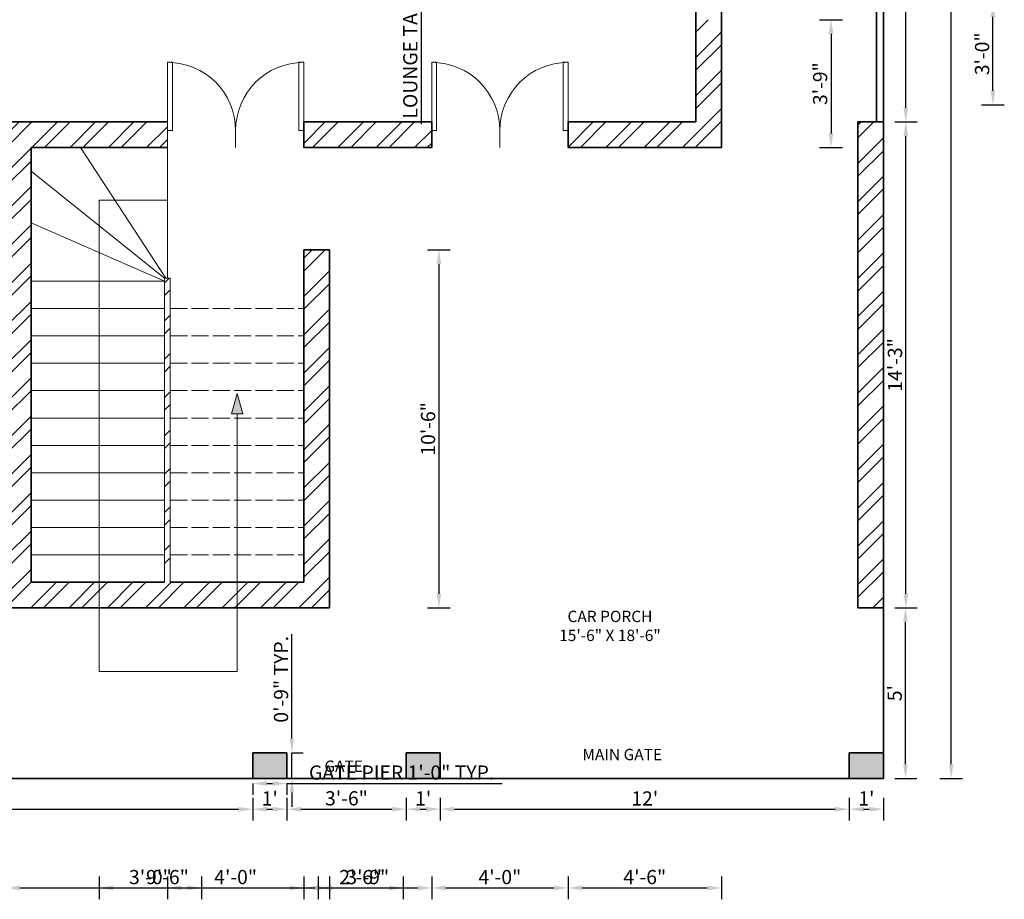
# Model space of a CAD drawing. Units: inches. Extents: x 468 to 1096, y 138 to 946.
# Tile 2 of 6: x 749 to 1096, y 139 to 448. Entities that reach past the tile are written whole.
import ezdxf

# ---------------------------------------------------------------- set-up
doc = ezdxf.new("R2010")
doc.units = ezdxf.units.IN
doc.linetypes.add('ACAD_ISO02W100', pattern=[15, 12, -3])
for name, color, linetype, lineweight in [('A-ANNO-DIMS', 2, 'Continuous', 18), ('A-ANNO-SYMB', 7, 'Continuous', 13), ('A-ANNO-TEXT', 7, 'Continuous', 18), ('A-AREA-IDEN', 7, 'Continuous', 18), ('A-DOOR', 3, 'Continuous', 18), ('A-FLOR-STRS', 7, 'Continuous', 18), ('A-FLOR-STRS-OVHD', 7, 'ACAD_ISO02W100', 18), ('A-SITE-GATE', 7, 'Continuous', 35), ('A-SITE-PATT', 8, 'Continuous', 13), ('A-WALL', 7, 'Continuous', 35), ('A-WALL-PATT', 8, 'Continuous', 13), ('C-PROP', 7, 'Continuous', 35)]:
    doc.layers.add(name, color=color, linetype=linetype, lineweight=lineweight)
doc.styles.get("Standard").update_dxf_attribs({"font": 'arial.ttf'})
doc.dimstyles.new('ISO-25', dxfattribs={"dimtxt": 5, "dimasz": 5, "dimexe": 4, "dimexo": 4, "dimtad": 1, "dimdec": 1, "dimlunit": 3, "dimtxsty": 'Standard', "dimcen": 2.5, "dimadec": 0, "dimazin": 0, "dimtfac": 1, "dimtdec": 1, "dimtmove": 0, "dimatfit": 3, "dimfxl": 4, "dimfxlon": 1, "dimarcsym": 0})

# ---------------------------------------------------------------- blocks, each defined once
blk = doc.blocks.new('*U5')
for p, q in [((-24, 0), (-24, -6)), ((0, 0), (0, -6))]:
    blk.add_line(p, q)
blk.add_lwpolyline([(0, 0), (0, 24), (-1.75, 24), (-1.75, 0)], close=True)
blk.add_arc((0, 0), 24, 90, 180)
blk = doc.blocks.new('*D19')
at = {"layer": 'A-ANNO-DIMS', "color": 0, "lineweight": -2, "transparency": 16777216}
for p, q in [((513.13, 174.32), (513.13, 166.32)), ((831.13, 174.32), (831.13, 166.32)), ((518.13, 170.32), (826.13, 170.32))]:
    blk.add_line(p, q, dxfattribs=at)
at = {"layer": 'A-ANNO-DIMS', "color": 0, "transparency": 16777216}
for points in [[(518.13, 171.15), (518.13, 169.48), (513.13, 170.32)], [(826.13, 171.15), (826.13, 169.48), (831.13, 170.32)]]:
    blk.add_solid(points, dxfattribs=at)
at = {"layer": 'Defpoints', "color": 0, "transparency": 16777216}
for p in [(513.13, 181.16), (831.13, 181.16), (831.13, 170.32)]:
    blk.add_point(p, dxfattribs=at)
at = {"layer": 'A-ANNO-DIMS', "color": 0, "transparency": 16777216, "insert": (672.13, 173.49), "char_height": 5, "attachment_point": 5}
blk.add_mtext('26\'-6"', dxfattribs=at)
blk = doc.blocks.new('*D20')
at = {"layer": 'A-ANNO-DIMS', "color": 0, "lineweight": -2, "transparency": 16777216}
for p, q in [((831.13, 174.32), (831.13, 166.32)), ((843.13, 174.32), (843.13, 166.32)), ((836.13, 170.32), (838.13, 170.32))]:
    blk.add_line(p, q, dxfattribs=at)
at = {"layer": 'A-ANNO-DIMS', "color": 0, "transparency": 16777216}
for points in [[(836.13, 171.15), (836.13, 169.48), (831.13, 170.32)], [(838.13, 171.15), (838.13, 169.48), (843.13, 170.32)]]:
    blk.add_solid(points, dxfattribs=at)
at = {"layer": 'Defpoints', "color": 0, "transparency": 16777216}
for p in [(831.13, 181.16), (843.13, 181.16), (843.13, 170.32)]:
    blk.add_point(p, dxfattribs=at)
at = {"layer": 'A-ANNO-DIMS', "color": 0, "transparency": 16777216, "insert": (837.13, 173.45), "char_height": 5, "attachment_point": 5}
blk.add_mtext("1'", dxfattribs=at)
blk = doc.blocks.new('*D21')
at = {"layer": 'A-ANNO-DIMS', "color": 0, "lineweight": -2, "transparency": 16777216}
for p, q in [((843.13, 174.32), (843.13, 166.32)), ((885.13, 174.32), (885.13, 166.32)), ((848.13, 170.32), (880.13, 170.32))]:
    blk.add_line(p, q, dxfattribs=at)
at = {"layer": 'A-ANNO-DIMS', "color": 0, "transparency": 16777216}
for points in [[(848.13, 171.15), (848.13, 169.48), (843.13, 170.32)], [(880.13, 171.15), (880.13, 169.48), (885.13, 170.32)]]:
    blk.add_solid(points, dxfattribs=at)
at = {"layer": 'Defpoints', "color": 0, "transparency": 16777216}
for p in [(843.13, 181.16), (885.13, 181.16), (885.13, 170.32)]:
    blk.add_point(p, dxfattribs=at)
at = {"layer": 'A-ANNO-DIMS', "color": 0, "transparency": 16777216, "insert": (864.13, 173.5), "char_height": 5, "attachment_point": 5}
blk.add_mtext('3\'-6"', dxfattribs=at)
blk = doc.blocks.new('*D22')
at = {"layer": 'A-ANNO-DIMS', "color": 0, "lineweight": -2, "transparency": 16777216}
for p, q in [((885.13, 174.32), (885.13, 166.32)), ((897.13, 174.32), (897.13, 166.32)), ((890.13, 170.32), (892.13, 170.32))]:
    blk.add_line(p, q, dxfattribs=at)
at = {"layer": 'A-ANNO-DIMS', "color": 0, "transparency": 16777216}
for points in [[(890.13, 171.15), (890.13, 169.48), (885.13, 170.32)], [(892.13, 171.15), (892.13, 169.48), (897.13, 170.32)]]:
    blk.add_solid(points, dxfattribs=at)
at = {"layer": 'Defpoints', "color": 0, "transparency": 16777216}
for p in [(885.13, 181.16), (897.13, 181.16), (897.13, 170.32)]:
    blk.add_point(p, dxfattribs=at)
at = {"layer": 'A-ANNO-DIMS', "color": 0, "transparency": 16777216, "insert": (891.13, 173.45), "char_height": 5, "attachment_point": 5}
blk.add_mtext("1'", dxfattribs=at)
blk = doc.blocks.new('*D23')
at = {"layer": 'A-ANNO-DIMS', "color": 0, "lineweight": -2, "transparency": 16777216}
for p, q in [((897.13, 174.32), (897.13, 166.32)), ((1041.13, 174.32), (1041.13, 166.32)), ((902.13, 170.32), (1036.13, 170.32))]:
    blk.add_line(p, q, dxfattribs=at)
at = {"layer": 'A-ANNO-DIMS', "color": 0, "transparency": 16777216}
for points in [[(902.13, 171.15), (902.13, 169.48), (897.13, 170.32)], [(1036.13, 171.15), (1036.13, 169.48), (1041.13, 170.32)]]:
    blk.add_solid(points, dxfattribs=at)
at = {"layer": 'Defpoints', "color": 0, "transparency": 16777216}
for p in [(897.13, 181.16), (1041.13, 181.16), (1041.13, 170.32)]:
    blk.add_point(p, dxfattribs=at)
at = {"layer": 'A-ANNO-DIMS', "color": 0, "transparency": 16777216, "insert": (969.13, 173.45), "char_height": 5, "attachment_point": 5}
blk.add_mtext("12'", dxfattribs=at)
blk = doc.blocks.new('*D24')
at = {"layer": 'A-ANNO-DIMS', "color": 0, "lineweight": -2, "transparency": 16777216}
for p, q in [((1041.13, 174.32), (1041.13, 166.32)), ((1053.13, 174.32), (1053.13, 166.32)), ((1046.13, 170.32), (1048.13, 170.32))]:
    blk.add_line(p, q, dxfattribs=at)
at = {"layer": 'A-ANNO-DIMS', "color": 0, "transparency": 16777216}
for points in [[(1046.13, 171.15), (1046.13, 169.48), (1041.13, 170.32)], [(1048.13, 171.15), (1048.13, 169.48), (1053.13, 170.32)]]:
    blk.add_solid(points, dxfattribs=at)
at = {"layer": 'Defpoints', "color": 0, "transparency": 16777216}
for p in [(1041.13, 181.16), (1053.13, 181.16), (1053.13, 170.32)]:
    blk.add_point(p, dxfattribs=at)
at = {"layer": 'A-ANNO-DIMS', "color": 0, "transparency": 16777216, "insert": (1047.13, 173.45), "char_height": 5, "attachment_point": 5}
blk.add_mtext("1'", dxfattribs=at)
blk = doc.blocks.new('*D25')
at = {"layer": 'A-ANNO-DIMS', "color": 0, "lineweight": -2, "transparency": 16777216}
for p, q in [((1057.13, 241.16), (1064.91, 241.16)), ((1060.91, 186.16), (1060.91, 236.16)), ((1057.13, 181.16), (1064.91, 181.16))]:
    blk.add_line(p, q, dxfattribs=at)
at = {"layer": 'A-ANNO-DIMS', "color": 0, "transparency": 16777216}
for points in [[(1060.07, 236.16), (1061.74, 236.16), (1060.91, 241.16)], [(1060.07, 186.16), (1061.74, 186.16), (1060.91, 181.16)]]:
    blk.add_solid(points, dxfattribs=at)
at = {"layer": 'Defpoints', "color": 0, "transparency": 16777216}
for p in [(1053.13, 241.16), (1060.91, 241.16), (1053.13, 181.16)]:
    blk.add_point(p, dxfattribs=at)
at = {"layer": 'A-ANNO-DIMS', "color": 0, "transparency": 16777216, "insert": (1057.74, 211.16), "char_height": 5, "attachment_point": 5, "rotation": 90}
blk.add_mtext("5'", dxfattribs=at)
blk = doc.blocks.new('*D26')
at = {"layer": 'A-ANNO-DIMS', "color": 0, "lineweight": -2, "transparency": 16777216}
for p, q in [((1073, 901.16), (1081, 901.16)), ((1077, 186.16), (1077, 896.16)), ((1073, 181.16), (1081, 181.16))]:
    blk.add_line(p, q, dxfattribs=at)
at = {"layer": 'A-ANNO-DIMS', "color": 0, "transparency": 16777216}
for points in [[(1076.17, 896.16), (1077.83, 896.16), (1077, 901.16)], [(1076.17, 186.16), (1077.83, 186.16), (1077, 181.16)]]:
    blk.add_solid(points, dxfattribs=at)
at = {"layer": 'Defpoints', "color": 0, "transparency": 16777216}
for p in [(1053.13, 901.16), (1077, 901.16), (1053.13, 181.16)]:
    blk.add_point(p, dxfattribs=at)
at = {"layer": 'A-ANNO-DIMS', "color": 0, "transparency": 16777216, "insert": (1073.82, 541.16), "char_height": 5, "attachment_point": 5, "rotation": 90}
blk.add_mtext("60'", dxfattribs=at)
blk = doc.blocks.new('*D27')
at = {"layer": 'A-ANNO-DIMS', "color": 0, "lineweight": -2, "transparency": 16777216}
for p, q in [((1057.13, 412.16), (1065.02, 412.16)), ((1061.02, 246.16), (1061.02, 407.16)), ((1057.13, 241.16), (1065.02, 241.16))]:
    blk.add_line(p, q, dxfattribs=at)
at = {"layer": 'A-ANNO-DIMS', "color": 0, "transparency": 16777216}
for points in [[(1060.18, 407.16), (1061.85, 407.16), (1061.02, 412.16)], [(1060.18, 246.16), (1061.85, 246.16), (1061.02, 241.16)]]:
    blk.add_solid(points, dxfattribs=at)
at = {"layer": 'Defpoints', "color": 0, "transparency": 16777216}
for p in [(1053.13, 412.16), (1061.02, 412.16), (1053.13, 241.16)]:
    blk.add_point(p, dxfattribs=at)
at = {"layer": 'A-ANNO-DIMS', "color": 0, "transparency": 16777216, "insert": (1057.84, 326.66), "char_height": 5, "attachment_point": 5, "rotation": 90}
blk.add_mtext('14\'-3"', dxfattribs=at)
blk = doc.blocks.new('*D28')
at = {"layer": 'A-ANNO-DIMS', "color": 0, "lineweight": -2, "transparency": 16777216}
for p, q in [((1057.13, 853.16), (1065.02, 853.16)), ((1061.02, 417.16), (1061.02, 848.16)), ((1057.13, 412.16), (1065.02, 412.16))]:
    blk.add_line(p, q, dxfattribs=at)
at = {"layer": 'A-ANNO-DIMS', "color": 0, "transparency": 16777216}
for points in [[(1060.18, 848.16), (1061.85, 848.16), (1061.02, 853.16)], [(1060.18, 417.16), (1061.85, 417.16), (1061.02, 412.16)]]:
    blk.add_solid(points, dxfattribs=at)
at = {"layer": 'Defpoints', "color": 0, "transparency": 16777216}
for p in [(1053.13, 853.16), (1061.02, 853.16), (1053.13, 412.16)]:
    blk.add_point(p, dxfattribs=at)
at = {"layer": 'A-ANNO-DIMS', "color": 0, "transparency": 16777216, "insert": (1057.84, 632.66), "char_height": 5, "attachment_point": 5, "rotation": 90}
blk.add_mtext('36\'-9"', dxfattribs=at)
blk = doc.blocks.new('GATE-PIER-12X9')
for p, q in [((0, 0), (0, 9)), ((0, 9), (12, 9)), ((12, 9), (12, 0))]:
    blk.add_line(p, q)
blk = doc.blocks.new('*D45')
at = {"layer": 'A-ANNO-DIMS', "color": 0, "lineweight": -2, "transparency": 16777216}
for p, q in [((831.13, 179.36), (831.13, 175.36)), ((836.13, 179.36), (838.13, 179.36)), ((843.13, 179.36), (843.13, 175.36)), ((843.13, 179.36), (918.98, 179.36))]:
    blk.add_line(p, q, dxfattribs=at)
at = {"layer": 'A-ANNO-DIMS', "color": 0, "transparency": 16777216}
for points in [[(836.13, 180.19), (836.13, 178.53), (831.13, 179.36)], [(838.13, 180.19), (838.13, 178.53), (843.13, 179.36)]]:
    blk.add_solid(points, dxfattribs=at)
at = {"layer": 'Defpoints', "color": 0, "transparency": 16777216}
for p in [(831.13, 181.16), (843.13, 181.16), (843.13, 179.36)]:
    blk.add_point(p, dxfattribs=at)
at = {"layer": 'A-ANNO-DIMS', "color": 0, "transparency": 16777216, "insert": (883.55, 182.57), "char_height": 5, "attachment_point": 5}
blk.add_mtext('GATE PIER 1\'-0" TYP.', dxfattribs=at)
blk = doc.blocks.new('*D46')
at = {"layer": 'A-ANNO-DIMS', "color": 0, "lineweight": -2, "transparency": 16777216}
for p, q in [((844.93, 195.16), (844.93, 231.89)), ((844.93, 190.16), (848.93, 190.16)), ((844.93, 181.16), (844.93, 190.16)), ((844.93, 181.16), (848.93, 181.16)), ((844.93, 176.16), (844.93, 171.16))]:
    blk.add_line(p, q, dxfattribs=at)
at = {"layer": 'A-ANNO-DIMS', "color": 0, "transparency": 16777216}
for points in [[(844.1, 195.16), (845.76, 195.16), (844.93, 190.16)], [(844.1, 176.16), (845.76, 176.16), (844.93, 181.16)]]:
    blk.add_solid(points, dxfattribs=at)
at = {"layer": 'Defpoints', "color": 0, "transparency": 16777216}
for p in [(843.13, 190.16), (844.93, 190.16), (843.13, 181.16)]:
    blk.add_point(p, dxfattribs=at)
at = {"layer": 'A-ANNO-DIMS', "color": 0, "transparency": 16777216, "insert": (841.75, 216.03), "char_height": 5, "attachment_point": 5, "rotation": 90}
blk.add_mtext('0\'-9" TYP.', dxfattribs=at)
blk = doc.blocks.new('*D51')
at = {"layer": 'A-ANNO-DIMS', "color": 0, "lineweight": -2, "transparency": 16777216}
for p, q in [((894.45, 546.23), (886.45, 546.23)), ((890.45, 541.23), (890.45, 491.23)), ((894.45, 486.23), (886.45, 486.23)), ((890.45, 486.23), (890.45, 411.4))]:
    blk.add_line(p, q, dxfattribs=at)
at = {"layer": 'A-ANNO-DIMS', "color": 0, "transparency": 16777216}
for points in [[(889.62, 541.23), (891.28, 541.23), (890.45, 546.23)], [(889.62, 491.23), (891.28, 491.23), (890.45, 486.23)]]:
    blk.add_solid(points, dxfattribs=at)
at = {"layer": 'Defpoints', "color": 0, "transparency": 16777216}
for p in [(899.45, 546.23), (890.45, 486.23), (899.45, 486.23)]:
    blk.add_point(p, dxfattribs=at)
at = {"layer": 'A-ANNO-DIMS', "color": 0, "transparency": 16777216, "insert": (887.24, 446.31), "char_height": 5, "attachment_point": 5, "rotation": 90}
blk.add_mtext('LOUNGE TABLE 5\'-0"', dxfattribs=at)
blk = doc.blocks.new('*D55')
at = {"layer": 'A-ANNO-DIMS', "color": 0, "lineweight": -2, "transparency": 16777216}
for p, q in [((744.13, 146.61), (744.13, 138.61)), ((858.13, 146.61), (858.13, 138.61)), ((749.13, 142.61), (853.13, 142.61))]:
    blk.add_line(p, q, dxfattribs=at)
at = {"layer": 'A-ANNO-DIMS', "color": 0, "transparency": 16777216}
for points in [[(749.13, 143.44), (749.13, 141.78), (744.13, 142.61)], [(853.13, 143.44), (853.13, 141.78), (858.13, 142.61)]]:
    blk.add_solid(points, dxfattribs=at)
at = {"layer": 'Defpoints', "color": 0, "transparency": 16777216}
for p in [(744.13, 241.16), (858.13, 241.16), (858.13, 142.61)]:
    blk.add_point(p, dxfattribs=at)
at = {"layer": 'A-ANNO-DIMS', "color": 0, "transparency": 16777216, "insert": (801.13, 145.79), "char_height": 5, "attachment_point": 5}
blk.add_mtext('9\'-6"', dxfattribs=at)
blk = doc.blocks.new('*D56')
at = {"layer": 'A-ANNO-DIMS', "color": 0, "lineweight": -2, "transparency": 16777216}
for p, q in [((892.68, 367.16), (900.68, 367.16)), ((896.68, 362.16), (896.68, 246.16)), ((892.68, 241.16), (900.68, 241.16))]:
    blk.add_line(p, q, dxfattribs=at)
at = {"layer": 'A-ANNO-DIMS', "color": 0, "transparency": 16777216}
for points in [[(895.85, 362.16), (897.51, 362.16), (896.68, 367.16)], [(895.85, 246.16), (897.51, 246.16), (896.68, 241.16)]]:
    blk.add_solid(points, dxfattribs=at)
at = {"layer": 'Defpoints', "color": 0, "transparency": 16777216}
for p in [(858.13, 367.16), (858.13, 241.16), (896.68, 241.16)]:
    blk.add_point(p, dxfattribs=at)
at = {"layer": 'A-ANNO-DIMS', "color": 0, "transparency": 16777216, "insert": (893.5, 304.16), "char_height": 5, "attachment_point": 5, "rotation": 90}
blk.add_mtext('10\'-6"', dxfattribs=at)
blk = doc.blocks.new('*D57')
at = {"layer": 'A-ANNO-DIMS', "color": 0, "lineweight": -2, "transparency": 16777216}
for p, q in [((801.13, 146.61), (801.13, 138.61)), ((849.13, 146.61), (849.13, 138.61)), ((806.13, 142.61), (844.13, 142.61))]:
    blk.add_line(p, q, dxfattribs=at)
at = {"layer": 'A-ANNO-DIMS', "color": 0, "transparency": 16777216}
for points in [[(806.13, 143.44), (806.13, 141.78), (801.13, 142.61)], [(844.13, 143.44), (844.13, 141.78), (849.13, 142.61)]]:
    blk.add_solid(points, dxfattribs=at)
at = {"layer": 'Defpoints', "color": 0, "transparency": 16777216}
for p in [(801.13, 403.16), (849.13, 403.16), (849.13, 142.61)]:
    blk.add_point(p, dxfattribs=at)
at = {"layer": 'A-ANNO-DIMS', "color": 0, "transparency": 16777216, "insert": (825.13, 145.79), "char_height": 5, "attachment_point": 5}
blk.add_mtext('4\'-0"', dxfattribs=at)
blk = doc.blocks.new('*D58')
at = {"layer": 'A-ANNO-DIMS', "color": 0, "lineweight": -2, "transparency": 16777216}
for p, q in [((849.13, 146.61), (849.13, 138.61)), ((894.13, 146.61), (894.13, 138.61)), ((854.13, 142.61), (889.13, 142.61))]:
    blk.add_line(p, q, dxfattribs=at)
at = {"layer": 'A-ANNO-DIMS', "color": 0, "transparency": 16777216}
for points in [[(854.13, 143.44), (854.13, 141.78), (849.13, 142.61)], [(889.13, 143.44), (889.13, 141.78), (894.13, 142.61)]]:
    blk.add_solid(points, dxfattribs=at)
at = {"layer": 'Defpoints', "color": 0, "transparency": 16777216}
for p in [(849.13, 403.16), (894.13, 403.16), (894.13, 142.61)]:
    blk.add_point(p, dxfattribs=at)
at = {"layer": 'A-ANNO-DIMS', "color": 0, "transparency": 16777216, "insert": (871.63, 145.79), "char_height": 5, "attachment_point": 5}
blk.add_mtext('3\'-9"', dxfattribs=at)
blk = doc.blocks.new('*D59')
at = {"layer": 'A-ANNO-DIMS', "color": 0, "lineweight": -2, "transparency": 16777216}
for p, q in [((894.13, 146.61), (894.13, 138.61)), ((942.13, 146.61), (942.13, 138.61)), ((899.13, 142.61), (937.13, 142.61))]:
    blk.add_line(p, q, dxfattribs=at)
at = {"layer": 'A-ANNO-DIMS', "color": 0, "transparency": 16777216}
for points in [[(899.13, 143.44), (899.13, 141.78), (894.13, 142.61)], [(937.13, 143.44), (937.13, 141.78), (942.13, 142.61)]]:
    blk.add_solid(points, dxfattribs=at)
at = {"layer": 'Defpoints', "color": 0, "transparency": 16777216}
for p in [(894.13, 403.16), (942.13, 403.16), (942.13, 142.61)]:
    blk.add_point(p, dxfattribs=at)
at = {"layer": 'A-ANNO-DIMS', "color": 0, "transparency": 16777216, "insert": (918.13, 145.79), "char_height": 5, "attachment_point": 5}
blk.add_mtext('4\'-0"', dxfattribs=at)
blk = doc.blocks.new('*D60')
at = {"layer": 'A-ANNO-DIMS', "color": 0, "lineweight": -2, "transparency": 16777216}
for p, q in [((942.13, 146.61), (942.13, 138.61)), ((996.13, 146.61), (996.13, 138.61)), ((947.13, 142.61), (991.13, 142.61))]:
    blk.add_line(p, q, dxfattribs=at)
at = {"layer": 'A-ANNO-DIMS', "color": 0, "transparency": 16777216}
for points in [[(947.13, 143.44), (947.13, 141.78), (942.13, 142.61)], [(991.13, 143.44), (991.13, 141.78), (996.13, 142.61)]]:
    blk.add_solid(points, dxfattribs=at)
at = {"layer": 'Defpoints', "color": 0, "transparency": 16777216}
for p in [(942.13, 403.16), (996.13, 403.16), (996.13, 142.61)]:
    blk.add_point(p, dxfattribs=at)
at = {"layer": 'A-ANNO-DIMS', "color": 0, "transparency": 16777216, "insert": (969.13, 145.79), "char_height": 5, "attachment_point": 5}
blk.add_mtext('4\'-6"', dxfattribs=at)
blk = doc.blocks.new('*D63')
at = {"layer": 'A-ANNO-DIMS', "color": 0, "lineweight": -2, "transparency": 16777216}
for p, q in [((777.13, 146.61), (777.13, 138.61)), ((813.13, 146.61), (813.13, 138.61)), ((782.13, 142.61), (808.13, 142.61))]:
    blk.add_line(p, q, dxfattribs=at)
at = {"layer": 'A-ANNO-DIMS', "color": 0, "transparency": 16777216}
for points in [[(782.13, 143.44), (782.13, 141.78), (777.13, 142.61)], [(808.13, 143.44), (808.13, 141.78), (813.13, 142.61)]]:
    blk.add_solid(points, dxfattribs=at)
at = {"layer": 'Defpoints', "color": 0, "transparency": 16777216}
for p in [(777.13, 682.16), (813.13, 682.16), (813.13, 142.61)]:
    blk.add_point(p, dxfattribs=at)
at = {"layer": 'A-ANNO-DIMS', "color": 0, "transparency": 16777216, "insert": (795.13, 145.79), "char_height": 5, "attachment_point": 5}
blk.add_mtext('3\'-0"', dxfattribs=at)
blk = doc.blocks.new('*D64')
at = {"layer": 'A-ANNO-DIMS', "color": 0, "lineweight": -2, "transparency": 16777216}
for p, q in [((854.13, 146.61), (854.13, 138.61)), ((884.13, 146.61), (884.13, 138.61)), ((859.13, 142.61), (879.13, 142.61))]:
    blk.add_line(p, q, dxfattribs=at)
at = {"layer": 'A-ANNO-DIMS', "color": 0, "transparency": 16777216}
for points in [[(859.13, 143.44), (859.13, 141.78), (854.13, 142.61)], [(879.13, 143.44), (879.13, 141.78), (884.13, 142.61)]]:
    blk.add_solid(points, dxfattribs=at)
at = {"layer": 'Defpoints', "color": 0, "transparency": 16777216}
for p in [(854.13, 766.16), (884.13, 766.16), (884.13, 142.61)]:
    blk.add_point(p, dxfattribs=at)
at = {"layer": 'A-ANNO-DIMS', "color": 0, "transparency": 16777216, "insert": (869.13, 145.79), "char_height": 5, "attachment_point": 5}
blk.add_mtext('2\'-6"', dxfattribs=at)
blk = doc.blocks.new('*D70')
at = {"layer": 'A-ANNO-DIMS', "color": 0, "lineweight": -2, "transparency": 16777216}
for p, q in [((1030.68, 448.16), (1038.68, 448.16)), ((1034.68, 443.16), (1034.68, 408.16)), ((1030.68, 403.16), (1038.68, 403.16))]:
    blk.add_line(p, q, dxfattribs=at)
at = {"layer": 'A-ANNO-DIMS', "color": 0, "transparency": 16777216}
for points in [[(1033.85, 443.16), (1035.51, 443.16), (1034.68, 448.16)], [(1033.85, 408.16), (1035.51, 408.16), (1034.68, 403.16)]]:
    blk.add_solid(points, dxfattribs=at)
at = {"layer": 'Defpoints', "color": 0, "transparency": 16777216}
for p in [(996.13, 448.16), (996.13, 403.16), (1034.68, 403.16)]:
    blk.add_point(p, dxfattribs=at)
at = {"layer": 'A-ANNO-DIMS', "color": 0, "transparency": 16777216, "insert": (1031.5, 425.66), "char_height": 5, "attachment_point": 5, "rotation": 90}
blk.add_mtext('3\'-9"', dxfattribs=at)
blk = doc.blocks.new('*D76')
at = {"layer": 'A-ANNO-DIMS', "color": 0, "lineweight": -2, "transparency": 16777216}
for p, q in [((1087.68, 454.16), (1095.68, 454.16)), ((1091.68, 423.16), (1091.68, 449.16)), ((1087.68, 418.16), (1095.68, 418.16))]:
    blk.add_line(p, q, dxfattribs=at)
at = {"layer": 'A-ANNO-DIMS', "color": 0, "transparency": 16777216}
for points in [[(1090.85, 449.16), (1092.51, 449.16), (1091.68, 454.16)], [(1090.85, 423.16), (1092.51, 423.16), (1091.68, 418.16)]]:
    blk.add_solid(points, dxfattribs=at)
at = {"layer": 'Defpoints', "color": 0, "transparency": 16777216}
for p in [(687.13, 454.16), (1091.68, 454.16), (687.13, 418.16)]:
    blk.add_point(p, dxfattribs=at)
at = {"layer": 'A-ANNO-DIMS', "color": 0, "transparency": 16777216, "insert": (1088.5, 436.16), "char_height": 5, "attachment_point": 5, "rotation": 90}
blk.add_mtext('3\'-0"', dxfattribs=at)

msp = doc.modelspace()

# ---------------------------------------------------------------- hatches: boundary and pattern name
at = {"layer": 'A-ANNO-SYMB'}
h = msp.add_hatch(color=256, dxfattribs=at)
h.dxf.hatch_style = 1
h.paths.add_polyline_path([(825.63, 316.65), (823.63, 309.43), (825.63, 309.43), (827.63, 309.43)])
at = {"layer": 'A-SITE-PATT'}
h = msp.add_hatch(color=256, dxfattribs=at)
h.dxf.hatch_style = 1
h.paths.add_polyline_path([(731.29, 185.66), (719.29, 185.66), (719.29, 181.16), (731.29, 181.16)])
h.paths.add_polyline_path([(843.13, 190.16), (831.13, 190.16), (831.13, 181.16), (843.13, 181.16)])
h.paths.add_polyline_path([(897.13, 190.16), (885.13, 190.16), (885.13, 181.16), (897.13, 181.16)])
h.paths.add_polyline_path([(1053.13, 190.16), (1041.13, 190.16), (1041.13, 181.16), (1053.13, 181.16)])
at = {"layer": 'A-WALL-PATT'}
h = msp.add_hatch(dxfattribs=at)
h.set_pattern_fill('ANSI32', color=256)
h.paths.add_polyline_path([(1053.13, 412.16), (1044.13, 412.16), (1044.13, 241.16), (1053.13, 241.16)])
h.paths.add_polyline_path([(996.13, 448.16), (987.13, 448.16), (987.13, 412.16), (942.13, 412.16), (942.13, 403.16), (996.13, 403.16)])
h.paths.add_polyline_path([(996.13, 532.16), (987.13, 532.16), (987.13, 496.16), (996.13, 496.16)])
h.paths.add_polyline_path([(996.13, 646.16), (987.13, 646.16), (987.13, 607.16), (813.13, 607.16), (813.13, 598.16), (822.13, 598.16), (987.13, 598.16), (987.13, 592.16), (996.13, 592.16), (996.13, 598.16), (996.13, 607.16)])
h.paths.add_polyline_path([(894.13, 412.16), (849.13, 412.16), (849.13, 403.16), (894.13, 403.16)])
h.paths.add_polyline_path([(801.13, 412.16), (744.13, 412.16), (744.13, 250.16), (744.13, 241.16), (777.13, 241.16), (777.13, 250.16), (753.13, 250.16), (753.13, 403.16), (801.13, 403.16)])
h.paths.add_polyline_path([(744.13, 412.16), (736.13, 412.16), (736.13, 403.16), (744.13, 403.16)])
h = msp.add_hatch(dxfattribs=at)
h.set_pattern_fill('ANSI32', color=256)
h.paths.add_polyline_path([(858.13, 367.16), (849.13, 367.16), (849.13, 250.16), (825.63, 250.16), (825.63, 241.16), (840.13, 241.16), (849.13, 241.16), (858.13, 241.16)])
h.paths.add_polyline_path([(825.63, 250.16), (802.13, 250.16), (802.13, 357.16), (800.13, 357.16), (800.13, 250.16), (777.13, 250.16), (777.13, 241.16), (825.63, 241.16)])

# ---------------------------------------------------------------- linework, layer by layer
at = {"layer": 'A-ANNO-SYMB'}
for p, q in [((801.13, 384.66), (777.13, 384.66)), ((777.13, 384.66), (777.13, 218.74)), ((823.63, 309.43), (825.63, 316.65)), ((827.63, 309.43), (825.63, 316.65)), ((825.63, 309.43), (823.63, 309.43)), ((825.63, 218.74), (825.63, 309.43)), ((825.63, 309.43), (827.63, 309.43)), ((777.13, 218.74), (825.63, 218.74))]:
    msp.add_line(p, q, dxfattribs=at)
at = {"layer": 'A-FLOR-STRS'}
for p, q in [((801.13, 357.16), (801.13, 412.16)), ((800.61, 357.16), (770.53, 403.16)), ((800.13, 357.16), (753.13, 394.88)), ((800.13, 356.16), (753.13, 376.68)), ((800.13, 357.16), (800.13, 250.16)), ((802.13, 357.16), (800.13, 357.16)), ((802.13, 357.16), (802.13, 250.16)), ((800.13, 356.16), (753.13, 356.16)), ((800.13, 346.53), (753.13, 346.53)), ((800.13, 336.89), (753.13, 336.89)), ((800.13, 327.26), (753.13, 327.26)), ((800.13, 317.62), (753.13, 317.62)), ((800.13, 307.98), (753.13, 307.98)), ((800.13, 298.35), (753.13, 298.35)), ((800.13, 288.71), (753.13, 288.71)), ((800.13, 279.08), (753.13, 279.08)), ((800.13, 269.44), (753.13, 269.44)), ((800.13, 259.81), (753.13, 259.81))]:
    msp.add_line(p, q, dxfattribs=at)
at = {"layer": 'A-FLOR-STRS-OVHD', "ltscale": 0.5}
for p, q in [((802.13, 346.53), (849.13, 346.53)), ((802.13, 336.89), (849.13, 336.89)), ((802.13, 327.26), (849.13, 327.26)), ((802.13, 317.62), (849.13, 317.62)), ((802.13, 307.98), (849.13, 307.98)), ((802.13, 298.35), (849.13, 298.35)), ((802.13, 288.71), (849.13, 288.71)), ((802.13, 279.08), (849.13, 279.08)), ((802.13, 269.44), (849.13, 269.44)), ((802.13, 259.81), (849.13, 259.81))]:
    msp.add_line(p, q, dxfattribs=at)
at = {"layer": 'A-SITE-GATE'}
for p, q in [((1041.13, 181.16), (1041.13, 190.16)), ((1041.13, 190.16), (1053.13, 190.16))]:
    msp.add_line(p, q, dxfattribs=at)
at = {"layer": 'A-WALL'}
for p, q in [((987.13, 412.16), (987.13, 598.16)), ((996.13, 403.16), (996.13, 598.16)), ((744.13, 412.16), (801.13, 412.16)), ((849.13, 412.16), (894.13, 412.16)), ((849.13, 403.16), (849.13, 412.16)), ((894.13, 403.16), (894.13, 412.16)), ((942.13, 403.16), (942.13, 412.16)), ((942.13, 412.16), (987.13, 412.16)), ((753.13, 403.16), (753.13, 250.16)), ((753.13, 403.16), (801.13, 403.16)), ((849.13, 403.16), (894.13, 403.16)), ((942.13, 403.16), (996.13, 403.16)), ((849.13, 250.16), (849.13, 367.16)), ((849.13, 367.16), (858.13, 367.16)), ((858.13, 241.16), (858.13, 367.16)), ((753.13, 250.16), (800.13, 250.16)), ((802.13, 250.16), (849.13, 250.16)), ((744.13, 241.16), (840.13, 241.16)), ((840.13, 241.16), (849.13, 241.16)), ((849.13, 241.16), (858.13, 241.16))]:
    msp.add_line(p, q, dxfattribs=at)
at = {"layer": 'C-PROP'}
for p, q in [((1053.13, 181.16), (1053.13, 901.16)), ((1050.72, 412.16), (1050.72, 892.16)), ((1044.13, 241.16), (1044.13, 412.16)), ((1044.13, 412.16), (1053.13, 412.16)), ((1044.13, 241.16), (1053.13, 241.16)), ((513.13, 181.16), (1053.13, 181.16))]:
    msp.add_line(p, q, dxfattribs=at)

# ---------------------------------------------------------------- block references
at = {"layer": 'A-DOOR', "xscale": -1}
for p in [(801.13, 409.16), (894.13, 409.16)]:
    msp.add_blockref('*U5', p, dxfattribs=at)
at = {"layer": 'A-DOOR'}
for p in [(849.13, 409.16), (942.13, 409.16)]:
    msp.add_blockref('*U5', p, dxfattribs=at)
at = {"layer": 'A-SITE-GATE'}
for p in [(831.13, 181.16), (885.13, 181.16)]:
    msp.add_blockref('GATE-PIER-12X9', p, dxfattribs=at)

# ---------------------------------------------------------------- texts
at = {"layer": 'A-ANNO-TEXT', "char_height": 4, "attachment_point": 1}
for s, insert in [('\\pxqc;MAIN GATE', (943.07, 191.56)), ('\\pxqc;GATE', (845.02, 187.44))]:
    msp.add_mtext_dynamic_manual_height_columns(s, width=36.2598, gutter_width=12.5, heights=[0], dxfattribs=dict(at, insert=insert))
at = {"layer": 'A-AREA-IDEN', "insert": (938.75, 240.16), "char_height": 4, "attachment_point": 1}
msp.add_mtext_dynamic_manual_height_columns('\\pxqc;CAR PORCH\\P15\'-6" X 18\'-6"', width=36.2598, gutter_width=12.5, heights=[0], dxfattribs=at)

# ---------------------------------------------------------------- dimensions: what is measured, and where the dimension line sits
at = {"layer": 'A-ANNO-DIMS'}
for base, p1, p2, angle, override, picture, middle in [((1077, 901.16), (1053.13, 181.16), (1053.13, 901.16), 90, {"dimclrd": 0, "dimclre": 0, "dimclrt": 0}, '*D26', (1073.82, 541.16)), ((1061.02, 853.16), (1053.13, 412.16), (1053.13, 853.16), 90, {"dimclrd": 0, "dimclre": 0, "dimclrt": 0}, '*D28', (1057.84, 632.66)), ((1091.68, 454.16), (687.13, 418.16), (687.13, 454.16), 90, {"dimdec": 1, "dimlfac": 1, "dimrnd": 0, "dimzin": 1, "dimdsep": 46, "dimlunit": 4, "dimfrac": 2}, '*D76', (1088.5, 436.16)), ((1034.68, 403.16), (996.13, 448.16), (996.13, 403.16), 270, {"dimdec": 1, "dimlfac": 1, "dimrnd": 0, "dimzin": 1, "dimdsep": 46, "dimlunit": 4, "dimfrac": 2}, '*D70', (1031.5, 425.66)), ((1061.02, 412.16), (1053.13, 241.16), (1053.13, 412.16), 90, {"dimclrd": 0, "dimclre": 0, "dimclrt": 0}, '*D27', (1057.84, 326.66)), ((896.68, 241.16), (858.13, 367.16), (858.13, 241.16), 270, {"dimdec": 1, "dimlfac": 1, "dimrnd": 0, "dimzin": 1, "dimdsep": 46, "dimlunit": 4, "dimfrac": 2}, '*D56', (893.5, 304.16)), ((1060.91, 241.16), (1053.13, 181.16), (1053.13, 241.16), 90, {"dimclrd": 0, "dimclre": 0, "dimclrt": 0}, '*D25', (1057.74, 211.16))]:
    dim = msp.add_linear_dim(base=base, p1=p1, p2=p2, angle=angle, dimstyle='ISO-25', override=override, dxfattribs=at)
    dim.commit()
    dim.dimension.update_dxf_attribs({"geometry": picture, "text_midpoint": middle})
for base, p1, p2, override, picture, middle in [((884.13, 142.61), (854.13, 766.16), (884.13, 766.16), {"dimdec": 1, "dimlfac": 1, "dimrnd": 0, "dimzin": 1, "dimdsep": 46, "dimlunit": 4, "dimfrac": 2}, '*D64', (869.13, 145.79)), ((813.13, 142.61), (777.13, 682.16), (813.13, 682.16), {"dimdec": 1, "dimlfac": 1, "dimrnd": 0, "dimzin": 1, "dimdsep": 46, "dimlunit": 4, "dimfrac": 2}, '*D63', (795.13, 145.79)), ((849.13, 142.61), (801.13, 403.16), (849.13, 403.16), {"dimdec": 1, "dimlfac": 1, "dimrnd": 0, "dimzin": 1, "dimdsep": 46, "dimlunit": 4, "dimfrac": 2}, '*D57', (825.13, 145.79)), ((894.13, 142.61), (849.13, 403.16), (894.13, 403.16), {"dimdec": 1, "dimlfac": 1, "dimrnd": 0, "dimzin": 1, "dimdsep": 46, "dimlunit": 4, "dimfrac": 2}, '*D58', (871.63, 145.79)), ((942.13, 142.61), (894.13, 403.16), (942.13, 403.16), {"dimdec": 1, "dimlfac": 1, "dimrnd": 0, "dimzin": 1, "dimdsep": 46, "dimlunit": 4, "dimfrac": 2}, '*D59', (918.13, 145.79)), ((996.13, 142.61), (942.13, 403.16), (996.13, 403.16), {"dimdec": 1, "dimlfac": 1, "dimrnd": 0, "dimzin": 1, "dimdsep": 46, "dimlunit": 4, "dimfrac": 2}, '*D60', (969.13, 145.79)), ((858.13, 142.61), (744.13, 241.16), (858.13, 241.16), {"dimdec": 1, "dimlfac": 1, "dimrnd": 0, "dimzin": 1, "dimdsep": 46, "dimlunit": 4, "dimfrac": 2}, '*D55', (801.13, 145.79)), ((831.13, 170.32), (513.13, 181.16), (831.13, 181.16), {"dimclrd": 0, "dimclre": 0, "dimclrt": 0}, '*D19', (672.13, 173.49)), ((843.13, 170.32), (831.13, 181.16), (843.13, 181.16), {"dimclrd": 0, "dimclre": 0, "dimclrt": 0, "dimtmove": 1}, '*D20', (837.13, 173.45)), ((885.13, 170.32), (843.13, 181.16), (885.13, 181.16), {"dimclrd": 0, "dimclre": 0, "dimclrt": 0, "dimtmove": 1}, '*D21', (864.13, 173.5)), ((897.13, 170.32), (885.13, 181.16), (897.13, 181.16), {"dimclrd": 0, "dimclre": 0, "dimclrt": 0, "dimtmove": 1}, '*D22', (891.13, 173.45)), ((1041.13, 170.32), (897.13, 181.16), (1041.13, 181.16), {"dimclrd": 0, "dimclre": 0, "dimclrt": 0, "dimtmove": 1}, '*D23', (969.13, 173.45)), ((1053.13, 170.32), (1041.13, 181.16), (1053.13, 181.16), {"dimclrd": 0, "dimclre": 0, "dimclrt": 0, "dimtmove": 1}, '*D24', (1047.13, 173.45))]:
    dim = msp.add_linear_dim(base=base, p1=p1, p2=p2, dimstyle='ISO-25', override=override, dxfattribs=at)
    dim.commit()
    dim.dimension.update_dxf_attribs({"geometry": picture, "text_midpoint": middle})
for base, p1, p2, angle, text, picture, middle in [((890.45, 486.23), (899.45, 546.23), (899.45, 486.23), 270, 'LOUNGE TABLE <>', '*D51', (887.24, 446.31)), ((844.93, 190.16), (843.13, 181.16), (843.13, 190.16), 90, '<> TYP.', '*D46', (841.75, 216.03))]:
    dim = msp.add_linear_dim(base=base, p1=p1, p2=p2, angle=angle, text=text, dimstyle='ISO-25', override={"dimdec": 1, "dimlfac": 1, "dimrnd": 0, "dimzin": 1, "dimdsep": 46, "dimlunit": 4, "dimfrac": 2}, dxfattribs=at)
    dim.commit()
    dim.dimension.update_dxf_attribs({"geometry": picture, "text_midpoint": middle})
dim = msp.add_linear_dim(base=(843.13, 179.36), p1=(831.13, 181.16), p2=(843.13, 181.16), text='GATE PIER <> TYP.', dimstyle='ISO-25', override={"dimdec": 1, "dimlfac": 1, "dimrnd": 0, "dimzin": 1, "dimdsep": 46, "dimlunit": 4, "dimfrac": 2}, dxfattribs=at)
dim.commit()
dim.dimension.update_dxf_attribs({"geometry": '*D45', "text_midpoint": (883.55, 182.57)})

doc.saveas('drawing.dxf')
